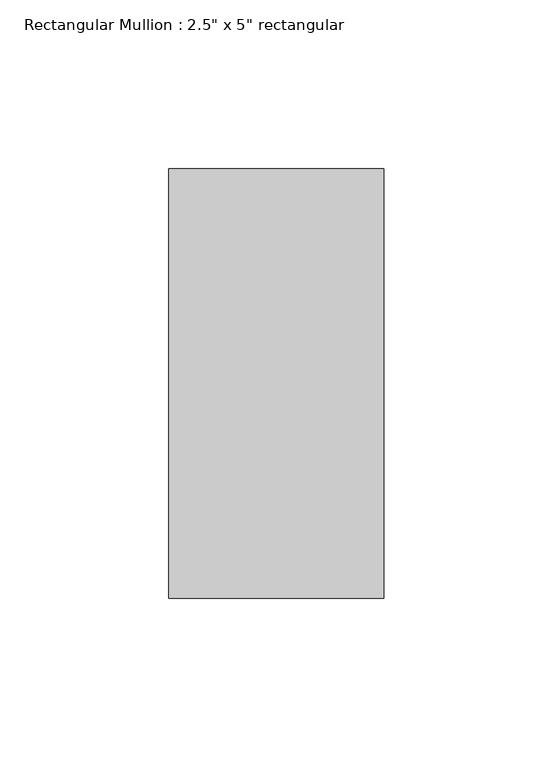
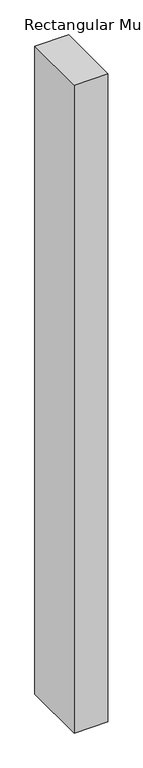
"""IFC4 building model written with IfcOpenShell, lengths in millimetres: member geometry."""

from ifc_helpers import new_model, si_unit, frame, origin, place, context, project, spatial, polyline, outline, extrude, source, transform, mapped, element, save


def member_5783932f(model_context):
    return source(origin(), model_context, "Body", "SweptSolid", [
        extrude(outline(polyline([(0.0, 63.5), (0.0, -63.5), (-63.5, -63.5), (-63.5, 63.5), (0.0, 63.5)])), frame((0.0, 0.0, -1282.7), z_axis=(0.0, 0.0, 1.0), x_axis=(1.0, 0.0, 0.0)), (0.0, 0.0, 1.0), 1282.7),
    ])


if __name__ == "__main__":
    model = new_model("IFC4")
    model_context = context("Model", 3, world=origin())
    ifc_project = project(units=[si_unit("LENGTHUNIT", "METRE", prefix="MILLI")], contexts=[model_context])
    site = spatial("IfcSite", under=ifc_project)
    building = spatial("IfcBuilding", under=site)
    placement = place(None, origin())
    member_shape = member_5783932f(model_context)
    element("IfcMember", 1, ObjectType="Rectangular Mullion : 2.5\" x 5\" rectangular", at=placement, inside=building, context=model_context, shape_type="MappedRepresentation", body=[
        mapped(member_shape, transform((0.0, 0.0, 0.0), x_axis=(1.0, 0.0, 0.0), y_axis=(0.0, 1.0, 0.0), z_axis=(0.0, 0.0, 1.0))),
    ])
    save(model, "model.ifc")

# Revit data of these elements
# Type "Rectangular Mullion : 2.5\" x 5\" rectangular"
#   built-in parameter 1007304 = 0.416667 (stored number, unit not read)
#   built-in parameter 1007301 = 0.104167 (stored number, unit not read)
#   built-in parameter 1007300 = 0.104167 (stored number, unit not read)
# Element 1 (IfcMember, "Rectangular Mullion : 2.5\" x 5\" rectangular")
#   Materials on its faces: "Aluminum"
# Materials
#   "Aluminum": class "Metal", colour RGB 247 247 247, transparency 0, Description = "Aluminum 6061", Cost = 0
